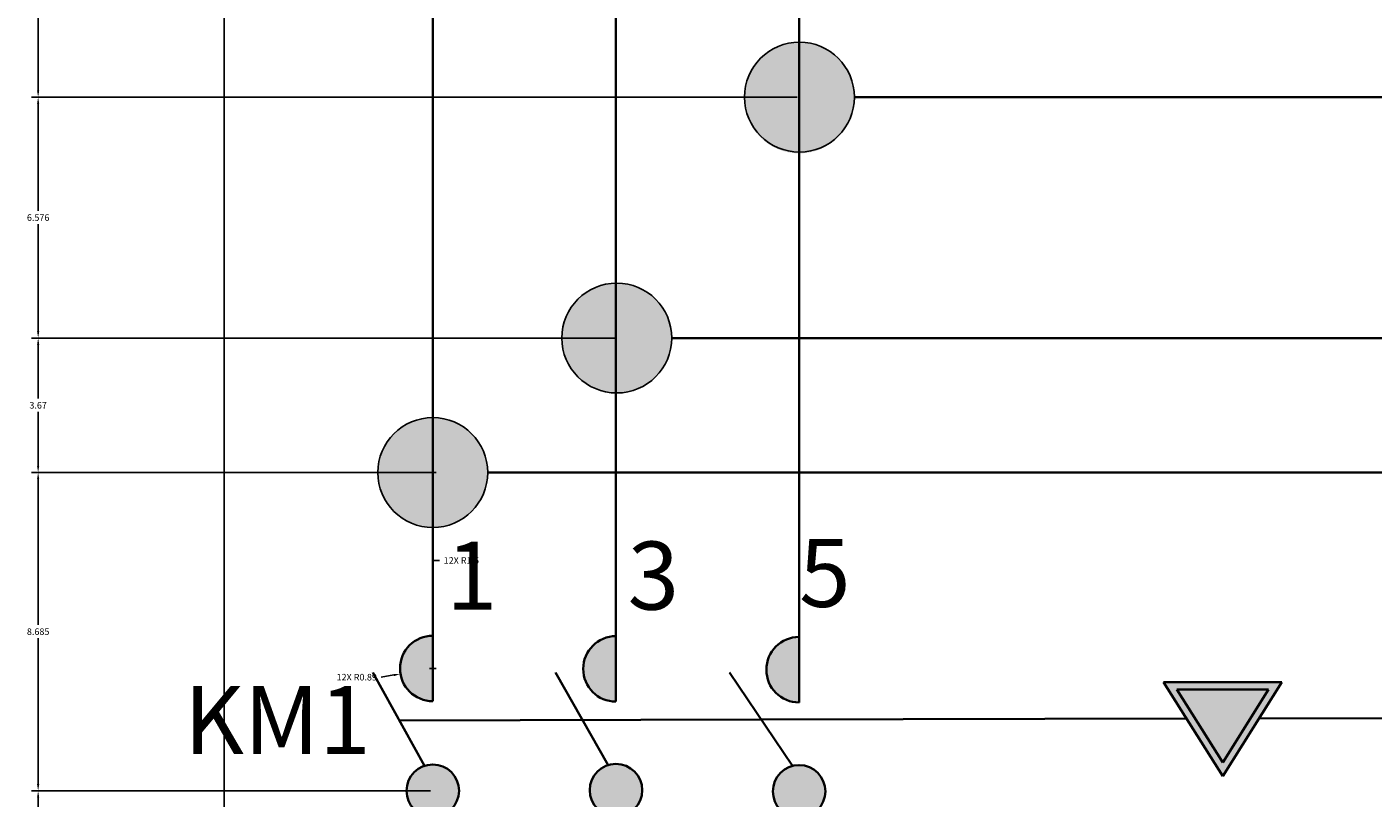
# Model space of a CAD drawing. Units: inches. Extents: x 237 to 313, y 343 to 451.
# Tile 3 of 6: x 237 to 274, y 410 to 431. Entities that reach past the tile are written whole.
import ezdxf

# ---------------------------------------------------------------- set-up
doc = ezdxf.new("R2010")
doc.units = ezdxf.units.IN
doc.header["$MEASUREMENT"] = 0
doc.layers.get('0').update_dxf_attribs({"color": 240})
for name, color, linetype, lineweight in [('A-ANNO-DIMS', 2, 'Continuous', 18), ('E-ANNO-TEXT', 7, 'Continuous', 25), ('E-DEVC', 4, 'Continuous', 35), ('E-PATT', 8, 'Continuous', 13), ('E-WIRE', 7, 'Continuous', 35), ('E-WIRE-JUNC', 7, 'Continuous', 25)]:
    doc.layers.add(name, color=color, linetype=linetype, lineweight=lineweight)
doc.styles.get("Standard").update_dxf_attribs({"font": 'arial.ttf'})
doc.dimstyles.get("Standard").update_dxf_attribs({"dimtxt": 0.18, "dimasz": 0.18, "dimexe": 0.18, "dimexo": 0.0625, "dimgap": 0.09, "dimtad": 0, "dimtih": 1, "dimtoh": 1, "dimdec": 4, "dimzin": 0, "dimdsep": 46, "dimtxsty": 'Standard', "dimcen": 0.09, "dimadec": 0, "dimazin": 0, "dimtfac": 1, "dimtdec": 4, "dimtofl": 0, "dimtmove": 0, "dimatfit": 3, "dimfxl": 1, "dimtolj": 1, "dimtzin": 0, "dimarcsym": 0})

# ---------------------------------------------------------------- blocks, each defined once
blk = doc.blocks.new('CONTACTOR-3P-NO')
h = blk.add_hatch(color=256)
h.dxf.hatch_style = 1
h.paths.add_polyline_path([(1.637, 4.965, 1), (1.637, 3.177)])
h.paths.add_polyline_path([(6.637, 4.953, 1), (6.637, 3.166)])
h.paths.add_polyline_path([(11.637, 4.931, 1), (11.637, 3.144)])
h = blk.add_hatch(color=256)
h.dxf.hatch_style = 1
h.paths.add_polyline_path([(2.354, 0.734, 1), (0.92, 0.734, 1)])
h.paths.add_polyline_path([(5.92, 0.749, 1), (7.354, 0.749, 1)])
h.paths.add_polyline_path([(10.92, 0.717, 1), (12.354, 0.717, 1)])
for p, q in [((1.414, 1.415), (0, 3.965)), ((6.423, 1.433), (4.991, 3.965)), ((11.461, 1.412), (9.739, 3.965))]:
    blk.add_line(p, q)
for centre in [(1.637, 0.734), (6.637, 0.749), (11.637, 0.717)]:
    blk.add_circle(centre, 0.717)
for centre in [(1.637, 4.071), (6.637, 4.06), (11.637, 4.037)]:
    blk.add_arc(centre, 0.894, 90, 270)
blk = doc.blocks.new('*D3')
at = {"layer": 'A-ANNO-DIMS', "color": 0, "lineweight": -2, "transparency": 16777216}
for p, q in [((242.3, 363.785), (242.3, 451.078)), ((242.48, 450.898), (274.084, 450.898)), ((306.476, 450.898), (274.872, 450.898)), ((306.656, 382.738), (306.656, 451.078))]:
    blk.add_line(p, q, dxfattribs=at)
at = {"layer": 'A-ANNO-DIMS', "color": 0, "lineweight": 35, "transparency": 16777216}
for points in [[(242.48, 450.928), (242.48, 450.868), (242.3, 450.898)], [(306.476, 450.928), (306.476, 450.868), (306.656, 450.898)]]:
    blk.add_solid(points, dxfattribs=at)
at = {"layer": 'Defpoints', "color": 0, "lineweight": 35, "transparency": 16777216}
for p in [(306.656, 450.898), (306.656, 382.675), (242.3, 363.723)]:
    blk.add_point(p, dxfattribs=at)
at = {"layer": 'A-ANNO-DIMS', "color": 0, "transparency": 16777216, "insert": (274.478, 450.898), "char_height": 0.18, "attachment_point": 5}
blk.add_mtext('\\A1;64.36', dxfattribs=at)
blk = doc.blocks.new('*D4')
at = {"layer": 'A-ANNO-DIMS', "color": 0, "lineweight": -2, "transparency": 16777216}
for p, q in [((258.115, 445.823), (312.65, 445.823)), ((312.47, 445.643), (312.47, 397.21)), ((312.47, 348.414), (312.47, 396.846)), ((289.124, 348.234), (312.65, 348.234))]:
    blk.add_line(p, q, dxfattribs=at)
at = {"layer": 'A-ANNO-DIMS', "color": 0, "lineweight": 35, "transparency": 16777216}
for points in [[(312.44, 445.643), (312.5, 445.643), (312.47, 445.823)], [(312.44, 348.414), (312.5, 348.414), (312.47, 348.234)]]:
    blk.add_solid(points, dxfattribs=at)
at = {"layer": 'Defpoints', "color": 0, "lineweight": 35, "transparency": 16777216}
for p in [(258.052, 445.823), (289.062, 348.234), (312.47, 348.234)]:
    blk.add_point(p, dxfattribs=at)
at = {"layer": 'A-ANNO-DIMS', "color": 0, "transparency": 16777216, "insert": (312.47, 397.028), "char_height": 0.18, "attachment_point": 5}
blk.add_mtext('\\A1;97.59', dxfattribs=at)
blk = doc.blocks.new('*D7')
at = {"layer": 'A-ANNO-DIMS', "color": 0, "lineweight": -2, "transparency": 16777216}
for p, q in [((257.997, 436.662), (257.997, 451.078)), ((258.177, 450.898), (269.926, 450.898)), ((282.468, 450.898), (270.718, 450.898)), ((282.648, 418.461), (282.648, 451.078))]:
    blk.add_line(p, q, dxfattribs=at)
at = {"layer": 'A-ANNO-DIMS', "color": 0, "lineweight": 35, "transparency": 16777216}
for points in [[(258.177, 450.928), (258.177, 450.868), (257.997, 450.898)], [(282.468, 450.928), (282.468, 450.868), (282.648, 450.898)]]:
    blk.add_solid(points, dxfattribs=at)
at = {"layer": 'Defpoints', "color": 0, "lineweight": 35, "transparency": 16777216}
for p in [(282.648, 450.898), (257.997, 436.599), (282.648, 418.399)]:
    blk.add_point(p, dxfattribs=at)
at = {"layer": 'A-ANNO-DIMS', "color": 0, "transparency": 16777216, "insert": (270.322, 450.898), "char_height": 0.18, "attachment_point": 5}
blk.add_mtext('\\A1;24.65', dxfattribs=at)
blk = doc.blocks.new('*D26')
at = {"layer": 'A-ANNO-DIMS', "color": 0, "lineweight": -2, "transparency": 16777216}
for p, q in [((247.934, 436.174), (237.045, 436.174)), ((237.225, 435.994), (237.225, 432.592)), ((237.225, 428.826), (237.225, 432.228)), ((257.943, 428.646), (237.045, 428.646))]:
    blk.add_line(p, q, dxfattribs=at)
at = {"layer": 'A-ANNO-DIMS', "color": 0, "lineweight": 35, "transparency": 16777216}
for points in [[(237.195, 435.994), (237.255, 435.994), (237.225, 436.174)], [(237.195, 428.826), (237.255, 428.826), (237.225, 428.646)]]:
    blk.add_solid(points, dxfattribs=at)
at = {"layer": 'Defpoints', "color": 0, "lineweight": 35, "transparency": 16777216}
for p in [(247.997, 436.174), (237.225, 428.646), (258.006, 428.646)]:
    blk.add_point(p, dxfattribs=at)
at = {"layer": 'A-ANNO-DIMS', "color": 0, "transparency": 16777216, "insert": (237.225, 432.41), "char_height": 0.18, "attachment_point": 5}
blk.add_mtext('\\A1;7.528', dxfattribs=at)
blk = doc.blocks.new('*D27')
at = {"layer": 'A-ANNO-DIMS', "color": 0, "lineweight": -2, "transparency": 16777216}
for p, q in [((257.943, 428.646), (237.045, 428.646)), ((237.225, 428.466), (237.225, 425.54)), ((237.225, 422.25), (237.225, 425.176)), ((252.956, 422.07), (237.045, 422.07))]:
    blk.add_line(p, q, dxfattribs=at)
at = {"layer": 'A-ANNO-DIMS', "color": 0, "lineweight": 35, "transparency": 16777216}
for points in [[(237.195, 428.466), (237.255, 428.466), (237.225, 428.646)], [(237.195, 422.25), (237.255, 422.25), (237.225, 422.07)]]:
    blk.add_solid(points, dxfattribs=at)
at = {"layer": 'Defpoints', "color": 0, "lineweight": 35, "transparency": 16777216}
for p in [(258.006, 428.646), (237.225, 422.07), (253.019, 422.07)]:
    blk.add_point(p, dxfattribs=at)
at = {"layer": 'A-ANNO-DIMS', "color": 0, "transparency": 16777216, "insert": (237.225, 425.358), "char_height": 0.18, "attachment_point": 5}
blk.add_mtext('\\A1;6.576', dxfattribs=at)
blk = doc.blocks.new('*D28')
at = {"layer": 'A-ANNO-DIMS', "color": 0, "lineweight": -2, "transparency": 16777216}
for p, q in [((252.956, 422.07), (237.045, 422.07)), ((237.225, 421.89), (237.225, 420.417)), ((237.225, 418.579), (237.225, 420.053)), ((247.934, 418.399), (237.045, 418.399))]:
    blk.add_line(p, q, dxfattribs=at)
at = {"layer": 'A-ANNO-DIMS', "color": 0, "lineweight": 35, "transparency": 16777216}
for points in [[(237.195, 421.89), (237.255, 421.89), (237.225, 422.07)], [(237.195, 418.579), (237.255, 418.579), (237.225, 418.399)]]:
    blk.add_solid(points, dxfattribs=at)
at = {"layer": 'Defpoints', "color": 0, "lineweight": 35, "transparency": 16777216}
for p in [(253.019, 422.07), (237.225, 418.399), (247.997, 418.399)]:
    blk.add_point(p, dxfattribs=at)
at = {"layer": 'A-ANNO-DIMS', "color": 0, "transparency": 16777216, "insert": (237.225, 420.235), "char_height": 0.18, "attachment_point": 5}
blk.add_mtext('\\A1;3.67', dxfattribs=at)
blk = doc.blocks.new('*D29')
at = {"layer": 'A-ANNO-DIMS', "color": 0, "lineweight": -2, "transparency": 16777216}
for p, q in [((247.934, 418.399), (237.045, 418.399)), ((237.225, 418.219), (237.225, 414.238)), ((237.225, 409.894), (237.225, 413.874)), ((247.934, 409.714), (237.045, 409.714))]:
    blk.add_line(p, q, dxfattribs=at)
at = {"layer": 'A-ANNO-DIMS', "color": 0, "lineweight": 35, "transparency": 16777216}
for points in [[(237.195, 418.219), (237.255, 418.219), (237.225, 418.399)], [(237.195, 409.894), (237.255, 409.894), (237.225, 409.714)]]:
    blk.add_solid(points, dxfattribs=at)
at = {"layer": 'Defpoints', "color": 0, "lineweight": 35, "transparency": 16777216}
for p in [(247.997, 418.399), (237.225, 409.714), (247.997, 409.714)]:
    blk.add_point(p, dxfattribs=at)
at = {"layer": 'A-ANNO-DIMS', "color": 0, "transparency": 16777216, "insert": (237.225, 414.056), "char_height": 0.18, "attachment_point": 5}
blk.add_mtext('\\A1;8.685', dxfattribs=at)
blk = doc.blocks.new('*D30')
at = {"layer": 'A-ANNO-DIMS', "color": 0, "lineweight": -2, "transparency": 16777216}
for p, q in [((247.934, 409.714), (237.045, 409.714)), ((237.225, 409.534), (237.225, 407.898)), ((237.225, 405.898), (237.225, 407.534)), ((257.934, 405.718), (237.045, 405.718))]:
    blk.add_line(p, q, dxfattribs=at)
at = {"layer": 'A-ANNO-DIMS', "color": 0, "lineweight": 35, "transparency": 16777216}
for points in [[(237.195, 409.534), (237.255, 409.534), (237.225, 409.714)], [(237.195, 405.898), (237.255, 405.898), (237.225, 405.718)]]:
    blk.add_solid(points, dxfattribs=at)
at = {"layer": 'Defpoints', "color": 0, "lineweight": 35, "transparency": 16777216}
for p in [(247.997, 409.714), (237.225, 405.718), (257.997, 405.718)]:
    blk.add_point(p, dxfattribs=at)
at = {"layer": 'A-ANNO-DIMS', "color": 0, "transparency": 16777216, "insert": (237.225, 407.716), "char_height": 0.18, "attachment_point": 5}
blk.add_mtext('\\A1;4.00', dxfattribs=at)
blk = doc.blocks.new('*D40')
at = {"layer": 'A-ANNO-DIMS', "color": 0, "lineweight": -2, "transparency": 16777216}
for p, q in [((247.907, 418.399), (248.087, 418.399)), ((247.997, 418.309), (247.997, 418.489)), ((248.002, 415.999), (248, 416.719)), ((248.182, 415.999), (248.002, 415.999))]:
    blk.add_line(p, q, dxfattribs=at)
at = {"layer": 'A-ANNO-DIMS', "color": 0, "lineweight": 35, "transparency": 16777216}
blk.add_solid([(248.03, 416.719), (247.97, 416.719), (248, 416.899)], dxfattribs=at)
at = {"layer": 'Defpoints', "color": 0, "lineweight": 35, "transparency": 16777216}
for p in [(247.997, 418.399), (248, 416.899)]:
    blk.add_point(p, dxfattribs=at)
at = {"layer": 'A-ANNO-DIMS', "color": 0, "transparency": 16777216, "insert": (248.777, 415.999), "char_height": 0.18, "attachment_point": 5}
blk.add_mtext('\\A1;12X R1.5', dxfattribs=at)
blk = doc.blocks.new('*D42')
at = {"layer": 'A-ANNO-DIMS', "color": 0, "lineweight": -2, "transparency": 16777216}
for p, q in [((247.907, 413.051), (248.087, 413.051)), ((247.997, 412.961), (247.997, 413.141)), ((246.587, 412.814), (246.938, 412.873))]:
    blk.add_line(p, q, dxfattribs=at)
at = {"layer": 'A-ANNO-DIMS', "color": 0, "lineweight": 35, "transparency": 16777216}
blk.add_solid([(246.933, 412.902), (246.943, 412.843), (247.116, 412.903)], dxfattribs=at)
at = {"layer": 'Defpoints', "color": 0, "lineweight": 35, "transparency": 16777216}
for p in [(247.997, 413.051), (247.116, 412.903)]:
    blk.add_point(p, dxfattribs=at)
at = {"layer": 'A-ANNO-DIMS', "color": 0, "transparency": 16777216, "insert": (245.922, 412.814), "char_height": 0.18, "attachment_point": 5}
blk.add_mtext('\\A1;12X R0.89', dxfattribs=at)

msp = doc.modelspace()

# ---------------------------------------------------------------- hatches: boundary and pattern name
at = {"layer": 'E-PATT'}
h = msp.add_hatch(color=256, dxfattribs=at)
h.dxf.hatch_style = 1
h.paths.add_polyline_path([(252.9994, 423.5586, 0.4142136), (251.4994, 422.0586, 0.4142136), (252.9994, 420.5586)])
h.paths.add_polyline_path([(254.4994, 422.0586, 0.4142136), (252.9994, 423.5586), (252.9994, 420.5586, 0.4142136)])
h.paths.add_polyline_path([(257.9994, 430.1098, 0.4142136), (256.4994, 428.6098, 0.4142136), (257.9994, 427.1098)])
h.paths.add_polyline_path([(259.4994, 428.6098, 0.4142136), (257.9994, 430.1098), (257.9994, 427.1098, 0.4142136)])
h = msp.add_hatch(color=256, dxfattribs=at)
h.dxf.hatch_style = 1
h.paths.add_polyline_path([(257.9968, 430.1459, 0.4124921), (256.5057, 428.6459, 0.4124921), (257.9968, 427.1459)])
h.paths.add_polyline_path([(257.9968, 430.1459), (257.9968, 427.1459, 0.4159371), (259.5057, 428.6459, 0.4159371)])
h = msp.add_hatch(color=256, dxfattribs=at)
h.dxf.hatch_style = 1
h.paths.add_polyline_path([(252.9968, 423.5702), (252.9968, 420.5705, 0.4184903), (254.5187, 422.0704, 0.4184903)])
h.paths.add_polyline_path([(252.9968, 423.5702, 0.4099497), (251.5187, 422.0704, 0.4099497), (252.9968, 420.5705)])
h = msp.add_hatch(color=256, dxfattribs=at)
h.dxf.hatch_style = 1
h.paths.add_polyline_path([(247.9968, 419.8988, 0.4142136), (246.4968, 418.3988, 0.4142136), (247.9968, 416.8988)])
h.paths.add_polyline_path([(247.9968, 419.8988), (247.9968, 416.8988, 0.4142136), (249.4968, 418.3988, 0.4142136)])
h = msp.add_hatch(color=256, dxfattribs=at)
h.dxf.hatch_style = 1
h.paths.add_polyline_path([(269.5638, 410.1118), (271.172, 412.6729), (270.8103, 412.6729), (268.3057, 412.6729), (267.9424, 412.6729)])
h.paths.add_polyline_path([(268.3057, 412.4729), (270.8103, 412.4729), (269.5631, 410.4868)], flags=16)
h = msp.add_hatch(color=256, dxfattribs=at)
h.dxf.hatch_style = 1
h.paths.add_polyline_path([(269.5631, 410.4868), (270.8103, 412.4729), (268.3057, 412.4729)])

# ---------------------------------------------------------------- linework, layer by layer
at = {"layer": 'E-DEVC'}
for p, q in [((269.5631, 410.1129), (267.9424, 412.6729)), ((268.3057, 412.6729), (267.9424, 412.6729)), ((268.3057, 412.6729), (270.8103, 412.6729)), ((271.172, 412.6729), (269.5631, 410.1107)), ((270.8103, 412.6729), (271.172, 412.6729)), ((268.3057, 412.4729), (270.8103, 412.4729)), ((269.5631, 410.4868), (268.3057, 412.4729)), ((270.8103, 412.4729), (269.5631, 410.4868)), ((247.0877, 411.6324), (256.9686, 411.6558)), ((256.9686, 411.6558), (268.5703, 411.6812)), ((270.552, 411.6855), (281.6957, 411.7099)), ((269.5631, 410.1129), (269.5631, 410.1107))]:
    msp.add_line(p, q, dxfattribs=at)
at = {"layer": 'E-WIRE'}
for p, q in [((252.9968, 435.9145), (252.9968, 418.3988)), ((257.9968, 435.8824), (257.9968, 418.3988)), ((247.9968, 435.4572), (247.9968, 416.8988)), ((259.5057, 428.6459), (292.6477, 428.6459)), ((254.5187, 422.0704), (287.6477, 422.0704)), ((247.9968, 418.3988), (247.9968, 412.1574)), ((249.4968, 418.3988), (282.6795, 418.3988)), ((252.9968, 418.3988), (252.9968, 412.1461)), ((257.9968, 418.3988), (257.9968, 412.1237))]:
    msp.add_line(p, q, dxfattribs=at)
at = {"layer": 'E-WIRE-JUNC'}
for points in [[(256.5057, 428.6459, 1), (259.5057, 428.6459, 1)], [(251.5187, 422.0704, 1), (254.5187, 422.0704, 1)], [(246.4968, 418.3988, 1), (249.4968, 418.3988, 1)]]:
    msp.add_lwpolyline(points, format="xyb", close=True, dxfattribs=at)

# ---------------------------------------------------------------- block references
at = {"layer": 'E-DEVC'}
msp.add_blockref('CONTACTOR-3P-NO', (246.36, 408.98), dxfattribs=at)

# ---------------------------------------------------------------- texts
at = {"layer": 'E-ANNO-TEXT'}
for s, height, p in [('1', 1.8564, (248.3582, 414.6575)), ('3', 1.8564, (253.3154, 414.6575)), ('5', 1.8564, (257.9968, 414.7316)), ('KM1', 1.85645, (241.2072, 410.7153))]:
    msp.add_text(s, height=height, dxfattribs=at).set_placement(p)

# ---------------------------------------------------------------- dimensions: what is measured, and where the dimension line sits
at = {"layer": 'A-ANNO-DIMS'}
for base, p1, p2, picture, middle in [((306.6564, 450.8976), (242.3002, 363.7227), (306.6564, 382.675), '*D3', (274.4783, 450.8976)), ((282.6477, 450.8976), (257.9968, 436.5992), (282.6477, 418.3988), '*D7', (270.3223, 450.8976))]:
    dim = msp.add_linear_dim(base=base, p1=p1, p2=p2, dimstyle='Standard', override={"dimdec": 2, "dimlfac": 1, "dimrnd": 0, "dimzin": 0, "dimdsep": 46, "dimlunit": 2}, dxfattribs=at)
    dim.commit()
    dim.dimension.update_dxf_attribs({"geometry": picture, "text_midpoint": middle})
for base, p1, p2, override, picture, middle in [((312.4701, 348.2337), (258.0525, 445.8226), (289.0615, 348.2337), {"dimdec": 2, "dimlfac": 1, "dimrnd": 0, "dimzin": 0, "dimdsep": 46, "dimlunit": 2}, '*D4', (312.4701, 397.0282)), ((237.2252, 428.6459), (247.9968, 436.1741), (258.0057, 428.6459), {"dimdec": 3, "dimlfac": 1, "dimrnd": 0, "dimzin": 0, "dimdsep": 46, "dimlunit": 2}, '*D26', (237.2252, 432.41)), ((237.22523, 422.07037), (258.00565, 428.64588), (253.0187, 422.07037), {"dimdec": 3, "dimlfac": 1, "dimrnd": 0, "dimzin": 0, "dimdsep": 46, "dimlunit": 2}, '*D27', (237.22523, 425.35812)), ((237.2252, 418.3988), (253.0187, 422.0704), (247.9968, 418.3988), {"dimdec": 2, "dimlfac": 1, "dimrnd": 0, "dimzin": 0, "dimdsep": 46, "dimlunit": 2}, '*D28', (237.2252, 420.2346)), ((237.2252, 409.7137), (247.9968, 418.3988), (247.9968, 409.7137), {"dimdec": 3, "dimlfac": 1, "dimrnd": 0, "dimzin": 0, "dimdsep": 46, "dimlunit": 2}, '*D29', (237.2252, 414.0563)), ((237.2252, 405.7183), (247.9968, 409.7137), (257.9968, 405.7183), {"dimdec": 2, "dimlfac": 1, "dimrnd": 0, "dimzin": 0, "dimdsep": 46, "dimlunit": 2}, '*D30', (237.2252, 407.716))]:
    dim = msp.add_linear_dim(base=base, p1=p1, p2=p2, angle=90, dimstyle='Standard', override=override, dxfattribs=at)
    dim.commit()
    dim.dimension.update_dxf_attribs({"geometry": picture, "text_midpoint": middle})
for center, mpoint, override, picture, middle in [((247.9968, 418.3988), (248, 416.8988), {"dimdec": 1, "dimlfac": 1, "dimrnd": 0, "dimzin": 0, "dimdsep": 46, "dimlunit": 2}, '*D40', (248.7774, 415.9988)), ((247.9968, 413.051), (247.1157, 412.9026), {"dimdec": 2, "dimlfac": 1, "dimrnd": 0, "dimzin": 0, "dimdsep": 46, "dimlunit": 2}, '*D42', (246.587, 412.8136))]:
    dim = msp.add_radius_dim(center=center, mpoint=mpoint, text='12X <>', dimstyle='Standard', override=override, dxfattribs=at)
    dim.commit()
    dim.dimension.update_dxf_attribs({"geometry": picture, "text_midpoint": middle, "dimtype": 164})

doc.saveas('drawing.dxf')
